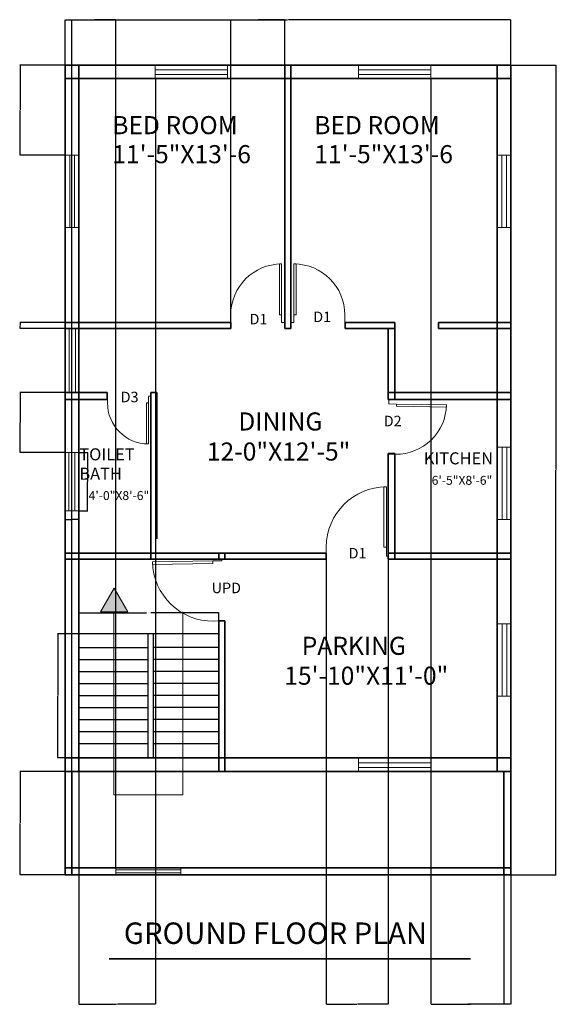
# Model space of a CAD drawing. Units: inches. Extents: x 2000 to 5103, y 1720 to 4295.
# Tile 1 of 2: x 2000 to 2357, y 1720 to 2374. Entities that reach past the tile are written whole.
import ezdxf

# ---------------------------------------------------------------- set-up
doc = ezdxf.new("R2010")
doc.units = ezdxf.units.IN
for name, color, linetype, lineweight in [('A-ANNO-DIMS', 2, 'Continuous', 18), ('A-ANNO-SYMB', 7, 'Continuous', 18), ('A-ANNO-TEXT', 3, 'Continuous', 18), ('A-ANNO-TITL', 7, 'Continuous', 35), ('A-AREA-IDEN', 7, 'Continuous', 25), ('A-DOOR', 4, 'Continuous', 18), ('A-WALL', 7, 'Continuous', 35), ('stair', 7, 'Continuous', 25), ('window', 10, 'Continuous', 18)]:
    doc.layers.add(name, color=color, linetype=linetype, lineweight=lineweight)
doc.styles.get("Standard").update_dxf_attribs({"font": 'arial.ttf'})
doc.dimstyles.get("Standard").update_dxf_attribs({"dimtxt": 0.18, "dimasz": 0.18, "dimexe": 0.18, "dimexo": 0.0625, "dimgap": 0.09, "dimtad": 0, "dimtih": 1, "dimtoh": 1, "dimdec": 4, "dimzin": 0, "dimdsep": 46, "dimtxsty": 'Standard', "dimcen": 0.09, "dimadec": 0, "dimazin": 0, "dimtfac": 1, "dimtdec": 4, "dimtofl": 0, "dimtmove": 0, "dimatfit": 3, "dimfxl": 1, "dimtolj": 1, "dimtzin": 0, "dimarcsym": 0})

# ---------------------------------------------------------------- blocks, each defined once
blk = doc.blocks.new('Dining Set - 36 x 72 in')
at = {"layer": 'window'}
for p, q in [((418.4, 887.02), (466.4, 887.02)), ((418.4, 883.92), (466.4, 883.92))]:
    blk.add_line(p, q, dxfattribs=at)
blk.add_lwpolyline([(418.4, 881.14), (418.4, 890.14), (466.4, 890.14), (466.4, 881.14)], close=True, dxfattribs=at)
blk = doc.blocks.new('*U3')
for p, q in [((0, 0), (0, -6)), ((40, 0), (40, -6))]:
    blk.add_line(p, q)
blk.add_lwpolyline([(0, 0), (0, 40), (1.75, 40), (1.75, 0)], close=True)
blk.add_arc((0, 0), 40, 0, 90)
blk = doc.blocks.new('WIN-DINING')
for p, q in [((2.68, 42.5), (2.68, 0)), ((4.5, 42.5), (4.5, 0)), ((6.78, 42.5), (6.78, 0))]:
    blk.add_line(p, q)
blk.add_lwpolyline([(0, 42.5), (9, 42.5), (9, 0), (0, 0)], close=True)
blk = doc.blocks.new('WIN-BATH')
for p, q in [((2.49, 38.59), (2.49, 0)), ((6.38, 38.59), (6.38, 0)), ((6.38, 38.59), (6.38, 0))]:
    blk.add_line(p, q)
blk.add_lwpolyline([(0, 38.59), (9, 38.59), (9, 0), (0, 0)], close=True)
blk = doc.blocks.new('WIN-FRONT')
for p, q in [((0, 3.25), (43.02, 3.25)), ((0, 1.25), (43.02, 1.25))]:
    blk.add_line(p, q)
blk.add_lwpolyline([(0, 4.5), (43.02, 4.5), (43.02, 0), (0, 0)], close=True)
blk = doc.blocks.new('STAIR-RETURN-FLIGHTS')
for p, q in [((93.06, 82.39), (0, 82.3)), ((46.1, 0), (46.1, 82.34)), ((49.5, 82.35), (49.5, 0)), ((0, 73.28), (46.1, 73.28)), ((49.5, 73.48), (93.06, 73.48)), ((49.5, 65.5), (93.06, 65.5)), ((0, 65.3), (46.1, 65.3)), ((0, 57.32), (46.1, 57.32)), ((49.5, 57.52), (93.06, 57.52)), ((0, 49.34), (46.1, 49.34)), ((49.5, 49.54), (93.06, 49.54)), ((0, 41.37), (46.1, 41.37)), ((49.5, 41.56), (93.06, 41.56)), ((0, 33.39), (46.1, 33.39)), ((49.5, 33.58), (93.06, 33.58)), ((0, 25.41), (46.1, 25.41)), ((49.5, 25.61), (93.06, 25.61)), ((0, 17.43), (46.1, 17.43)), ((49.5, 17.63), (93.06, 17.63)), ((0, 9.45), (46.1, 9.45)), ((49.5, 9.65), (93.06, 9.65))]:
    blk.add_line(p, q)
blk = doc.blocks.new('STAIR-PATH-ARROW')
h = blk.add_hatch(color=256)
h.dxf.hatch_style = 1
h.paths.add_polyline_path([(9.07, 137.14), (0, 121.43), (18.13, 121.43)])
for p, q in [((0, 121.43), (9.07, 137.14)), ((9.07, 137.14), (18.13, 121.43)), ((18.13, 121.43), (0, 121.43)), ((8.84, 0), (8.84, 121.43)), ((8.84, 121.43), (18.13, 121.43)), ((54.71, 121.43), (54.71, 0)), ((54.71, 0), (8.84, 0))]:
    blk.add_line(p, q)
blk = doc.blocks.new('*D13')
at = {"layer": 'A-ANNO-DIMS', "color": 0, "lineweight": -2, "transparency": 16777216}
for p, q in [((2039.72, 2086.19), (2045.62, 2086.19)), ((2045.44, 2086.01), (2045.44, 2067.07)), ((2045.44, 2047.77), (2045.44, 2066.71)), ((2039.72, 2047.59), (2045.62, 2047.59))]:
    blk.add_line(p, q, dxfattribs=at)
at = {"layer": 'A-ANNO-DIMS', "color": 0, "transparency": 16777216}
for points in [[(2045.41, 2086.01), (2045.47, 2086.01), (2045.44, 2086.19)], [(2045.41, 2047.77), (2045.47, 2047.77), (2045.44, 2047.59)]]:
    blk.add_solid(points, dxfattribs=at)
at = {"layer": 'Defpoints', "color": 0, "transparency": 16777216}
for p in [(2039.66, 2086.19), (2045.44, 2086.19), (2039.66, 2047.59)]:
    blk.add_point(p, dxfattribs=at)
at = {"layer": 'A-ANNO-DIMS', "color": 0, "transparency": 16777216, "insert": (2045.44, 2066.89), "char_height": 0.18, "attachment_point": 5}
blk.add_mtext('\\A1;WINDOW 39 TYP.', dxfattribs=at)
blk = doc.blocks.new('*D14')
at = {"layer": 'A-ANNO-DIMS', "color": 0, "lineweight": -2, "transparency": 16777216}
for p, q in [((2030.66, 2047.53), (2030.66, 2041.63)), ((2039.66, 2047.53), (2039.66, 2041.63)), ((2030.84, 2041.81), (2034.7, 2041.81)), ((2039.48, 2041.81), (2035.61, 2041.81))]:
    blk.add_line(p, q, dxfattribs=at)
at = {"layer": 'A-ANNO-DIMS', "color": 0, "transparency": 16777216}
for points in [[(2030.84, 2041.84), (2030.84, 2041.78), (2030.66, 2041.81)], [(2039.48, 2041.84), (2039.48, 2041.78), (2039.66, 2041.81)]]:
    blk.add_solid(points, dxfattribs=at)
at = {"layer": 'Defpoints', "color": 0, "transparency": 16777216}
for p in [(2030.66, 2047.59), (2039.66, 2047.59), (2039.66, 2041.81)]:
    blk.add_point(p, dxfattribs=at)
at = {"layer": 'A-ANNO-DIMS', "color": 0, "transparency": 16777216, "insert": (2035.16, 2041.81), "char_height": 0.18, "attachment_point": 5}
blk.add_mtext('\\A1;9 TYP.', dxfattribs=at)
blk = doc.blocks.new('*D17')
at = {"layer": 'A-ANNO-DIMS', "color": 0, "lineweight": -2, "transparency": 16777216}
for p, q in [((2039.66, 1965.97), (2039.66, 1980.04)), ((2039.84, 1979.86), (2084.7, 1979.86)), ((2132.54, 1979.86), (2087.67, 1979.86)), ((2132.72, 1965.97), (2132.72, 1980.04))]:
    blk.add_line(p, q, dxfattribs=at)
at = {"layer": 'A-ANNO-DIMS', "color": 0, "transparency": 16777216}
for points in [[(2039.84, 1979.89), (2039.84, 1979.83), (2039.66, 1979.86)], [(2132.54, 1979.89), (2132.54, 1979.83), (2132.72, 1979.86)]]:
    blk.add_solid(points, dxfattribs=at)
at = {"layer": 'Defpoints', "color": 0, "transparency": 16777216}
for p in [(2132.72, 1979.86), (2039.66, 1965.9), (2132.72, 1965.9)]:
    blk.add_point(p, dxfattribs=at)
at = {"layer": 'A-ANNO-DIMS', "color": 0, "transparency": 16777216, "insert": (2086.19, 1979.86), "char_height": 0.18, "attachment_point": 5}
blk.add_mtext('\\A1;RETURN STAIR 93 TYP.', dxfattribs=at)
blk = doc.blocks.new('*D18')
at = {"layer": 'A-ANNO-DIMS', "color": 0, "lineweight": -2, "transparency": 16777216}
for p, q in [((2039.59, 1965.9), (2025.52, 1965.9)), ((2025.7, 1965.72), (2025.7, 1924.89)), ((2025.7, 1883.69), (2025.7, 1924.53)), ((2039.59, 1883.51), (2025.52, 1883.51))]:
    blk.add_line(p, q, dxfattribs=at)
at = {"layer": 'A-ANNO-DIMS', "color": 0, "transparency": 16777216}
for points in [[(2025.67, 1965.72), (2025.73, 1965.72), (2025.7, 1965.9)], [(2025.67, 1883.69), (2025.73, 1883.69), (2025.7, 1883.51)]]:
    blk.add_solid(points, dxfattribs=at)
at = {"layer": 'Defpoints', "color": 0, "transparency": 16777216}
for p in [(2025.7, 1965.9), (2039.66, 1965.9), (2039.66, 1883.51)]:
    blk.add_point(p, dxfattribs=at)
at = {"layer": 'A-ANNO-DIMS', "color": 0, "transparency": 16777216, "insert": (2025.7, 1924.71), "char_height": 0.18, "attachment_point": 5}
blk.add_mtext('\\A1;82 TYP.', dxfattribs=at)
blk = doc.blocks.new('*D19')
at = {"layer": 'A-ANNO-DIMS', "color": 0, "lineweight": -2, "transparency": 16777216}
for p, q in [((2030.66, 2343.57), (2030.66, 2373.59)), ((2030.84, 2373.41), (2178.37, 2373.41)), ((2326.48, 2373.41), (2178.95, 2373.41)), ((2326.66, 2343.57), (2326.66, 2373.59))]:
    blk.add_line(p, q, dxfattribs=at)
at = {"layer": 'A-ANNO-DIMS', "color": 0, "transparency": 16777216}
for points in [[(2030.84, 2373.44), (2030.84, 2373.38), (2030.66, 2373.41)], [(2326.48, 2373.44), (2326.48, 2373.38), (2326.66, 2373.41)]]:
    blk.add_solid(points, dxfattribs=at)
at = {"layer": 'Defpoints', "color": 0, "transparency": 16777216}
for p in [(2326.66, 2373.41), (2030.66, 2343.51), (2326.66, 2343.51)]:
    blk.add_point(p, dxfattribs=at)
at = {"layer": 'A-ANNO-DIMS', "color": 0, "transparency": 16777216, "insert": (2178.66, 2373.41), "char_height": 0.18, "attachment_point": 5}
blk.add_mtext('\\A1;296', dxfattribs=at)
blk = doc.blocks.new('*D20')
at = {"layer": 'A-ANNO-DIMS', "color": 0, "lineweight": -2, "transparency": 16777216}
for p, q in [((2326.72, 2343.51), (2356.85, 2343.51)), ((2356.67, 2343.33), (2356.67, 2074.9)), ((2356.67, 1806.1), (2356.67, 2074.54)), ((2326.72, 1805.92), (2356.85, 1805.92))]:
    blk.add_line(p, q, dxfattribs=at)
at = {"layer": 'A-ANNO-DIMS', "color": 0, "transparency": 16777216}
for points in [[(2356.64, 2343.33), (2356.7, 2343.33), (2356.67, 2343.51)], [(2356.64, 1806.1), (2356.7, 1806.1), (2356.67, 1805.92)]]:
    blk.add_solid(points, dxfattribs=at)
at = {"layer": 'Defpoints', "color": 0, "transparency": 16777216}
for p in [(2326.66, 2343.51), (2356.67, 2343.51), (2326.66, 1805.92)]:
    blk.add_point(p, dxfattribs=at)
at = {"layer": 'A-ANNO-DIMS', "color": 0, "transparency": 16777216, "insert": (2356.67, 2074.72), "char_height": 0.18, "attachment_point": 5}
blk.add_mtext('\\A1;537.6', dxfattribs=at)
blk = doc.blocks.new('*D23')
at = {"layer": 'A-ANNO-DIMS', "color": 0, "lineweight": -2, "transparency": 16777216}
for p, q in [((2030.59, 1874.51), (2000.58, 1874.51)), ((2000.76, 1874.33), (2000.76, 1840.4)), ((2000.76, 1806.1), (2000.76, 1840.04)), ((2030.59, 1805.92), (2000.58, 1805.92))]:
    blk.add_line(p, q, dxfattribs=at)
at = {"layer": 'A-ANNO-DIMS', "color": 0, "transparency": 16777216}
for points in [[(2000.73, 1874.33), (2000.79, 1874.33), (2000.76, 1874.51)], [(2000.73, 1806.1), (2000.79, 1806.1), (2000.76, 1805.92)]]:
    blk.add_solid(points, dxfattribs=at)
at = {"layer": 'Defpoints', "color": 0, "transparency": 16777216}
for p in [(2000.76, 1874.51), (2030.66, 1874.51), (2030.66, 1805.92)]:
    blk.add_point(p, dxfattribs=at)
at = {"layer": 'A-ANNO-DIMS', "color": 0, "transparency": 16777216, "insert": (2000.76, 1840.22), "char_height": 0.18, "attachment_point": 5}
blk.add_mtext('\\A1;68.59', dxfattribs=at)
blk = doc.blocks.new('*D24')
at = {"layer": 'A-ANNO-DIMS', "color": 0, "lineweight": -2, "transparency": 16777216}
for p, q in [((2030.59, 2343.51), (2000.58, 2343.51)), ((2000.76, 2343.33), (2000.76, 2313.76)), ((2000.76, 2283.83), (2000.76, 2313.4)), ((2030.59, 2283.65), (2000.58, 2283.65))]:
    blk.add_line(p, q, dxfattribs=at)
at = {"layer": 'A-ANNO-DIMS', "color": 0, "transparency": 16777216}
for points in [[(2000.73, 2343.33), (2000.79, 2343.33), (2000.76, 2343.51)], [(2000.73, 2283.83), (2000.79, 2283.83), (2000.76, 2283.65)]]:
    blk.add_solid(points, dxfattribs=at)
at = {"layer": 'Defpoints', "color": 0, "transparency": 16777216}
for p in [(2030.66, 2343.51), (2000.76, 2283.65), (2030.66, 2283.65)]:
    blk.add_point(p, dxfattribs=at)
at = {"layer": 'A-ANNO-DIMS', "color": 0, "transparency": 16777216, "insert": (2000.76, 2313.58), "char_height": 0.18, "attachment_point": 5}
blk.add_mtext('\\A1;59.86', dxfattribs=at)
blk = doc.blocks.new('*D25')
at = {"layer": 'A-ANNO-DIMS', "color": 0, "lineweight": -2, "transparency": 16777216}
for p, q in [((2030.59, 2126.01), (2000.58, 2126.01)), ((2000.76, 2125.83), (2000.76, 2106.28)), ((2000.76, 2086.37), (2000.76, 2105.92)), ((2030.59, 2086.19), (2000.58, 2086.19))]:
    blk.add_line(p, q, dxfattribs=at)
at = {"layer": 'A-ANNO-DIMS', "color": 0, "transparency": 16777216}
for points in [[(2000.73, 2125.83), (2000.79, 2125.83), (2000.76, 2126.01)], [(2000.73, 2086.37), (2000.79, 2086.37), (2000.76, 2086.19)]]:
    blk.add_solid(points, dxfattribs=at)
at = {"layer": 'Defpoints', "color": 0, "transparency": 16777216}
for p in [(2030.66, 2126.01), (2000.76, 2086.19), (2030.66, 2086.19)]:
    blk.add_point(p, dxfattribs=at)
at = {"layer": 'A-ANNO-DIMS', "color": 0, "transparency": 16777216, "insert": (2000.76, 2106.1), "char_height": 0.18, "attachment_point": 5}
blk.add_mtext('\\A1;39.83', dxfattribs=at)
blk = doc.blocks.new('*D26')
at = {"layer": 'A-ANNO-DIMS', "color": 0, "lineweight": -2, "transparency": 16777216}
for p, q in [((2035.16, 1805.99), (2035.16, 2373.59)), ((2035.34, 2373.41), (2049.39, 2373.41)), ((2064.24, 2373.41), (2050.18, 2373.41)), ((2064.42, 1810.49), (2064.42, 2373.59))]:
    blk.add_line(p, q, dxfattribs=at)
at = {"layer": 'A-ANNO-DIMS', "color": 0, "transparency": 16777216}
for points in [[(2035.34, 2373.44), (2035.34, 2373.38), (2035.16, 2373.41)], [(2064.24, 2373.44), (2064.24, 2373.38), (2064.42, 2373.41)]]:
    blk.add_solid(points, dxfattribs=at)
at = {"layer": 'Defpoints', "color": 0, "transparency": 16777216}
for p in [(2064.42, 2373.41), (2035.16, 1805.92), (2064.42, 1810.42)]:
    blk.add_point(p, dxfattribs=at)
at = {"layer": 'A-ANNO-DIMS', "color": 0, "transparency": 16777216, "insert": (2049.79, 2373.41), "char_height": 0.18, "attachment_point": 5}
blk.add_mtext('\\A1;29.26', dxfattribs=at)
blk = doc.blocks.new('*D27')
at = {"layer": 'A-ANNO-DIMS', "color": 0, "lineweight": -2, "transparency": 16777216}
for p, q in [((2039.66, 2343.45), (2039.66, 1719.92)), ((2090.58, 2334.45), (2090.58, 1719.92)), ((2039.84, 1720.1), (2064.72, 1720.1)), ((2090.4, 1720.1), (2065.51, 1720.1))]:
    blk.add_line(p, q, dxfattribs=at)
at = {"layer": 'A-ANNO-DIMS', "color": 0, "transparency": 16777216}
for points in [[(2039.84, 1720.13), (2039.84, 1720.07), (2039.66, 1720.1)], [(2090.4, 1720.13), (2090.4, 1720.07), (2090.58, 1720.1)]]:
    blk.add_solid(points, dxfattribs=at)
at = {"layer": 'Defpoints', "color": 0, "transparency": 16777216}
for p in [(2039.66, 2343.51), (2090.58, 2334.51), (2090.58, 1720.1)]:
    blk.add_point(p, dxfattribs=at)
at = {"layer": 'A-ANNO-DIMS', "color": 0, "transparency": 16777216, "insert": (2065.12, 1720.1), "char_height": 0.18, "attachment_point": 5}
blk.add_mtext('\\A1;50.92', dxfattribs=at)
blk = doc.blocks.new('*D28')
at = {"layer": 'A-ANNO-DIMS', "color": 0, "lineweight": -2, "transparency": 16777216}
for p, q in [((2273.66, 2334.45), (2273.66, 1719.92)), ((2326.66, 2334.45), (2326.66, 1719.92)), ((2273.84, 1720.1), (2299.94, 1720.1)), ((2326.48, 1720.1), (2300.37, 1720.1))]:
    blk.add_line(p, q, dxfattribs=at)
at = {"layer": 'A-ANNO-DIMS', "color": 0, "transparency": 16777216}
for points in [[(2273.84, 1720.13), (2273.84, 1720.07), (2273.66, 1720.1)], [(2326.48, 1720.13), (2326.48, 1720.07), (2326.66, 1720.1)]]:
    blk.add_solid(points, dxfattribs=at)
at = {"layer": 'Defpoints', "color": 0, "transparency": 16777216}
for p in [(2273.66, 2334.51), (2326.66, 2334.51), (2326.66, 1720.1)]:
    blk.add_point(p, dxfattribs=at)
at = {"layer": 'A-ANNO-DIMS', "color": 0, "transparency": 16777216, "insert": (2300.16, 1720.1), "char_height": 0.18, "attachment_point": 5}
blk.add_mtext('\\A1;53', dxfattribs=at)
blk = doc.blocks.new('*D31')
at = {"layer": 'A-ANNO-DIMS', "color": 0, "lineweight": -2, "transparency": 16777216}
for p, q in [((2273.66, 1874.36), (2273.66, 1719.92)), ((2322.16, 1874.45), (2322.16, 1719.92)), ((2273.84, 1720.1), (2297.58, 1720.1)), ((2321.98, 1720.1), (2298.23, 1720.1))]:
    blk.add_line(p, q, dxfattribs=at)
at = {"layer": 'A-ANNO-DIMS', "color": 0, "transparency": 16777216}
for points in [[(2273.84, 1720.13), (2273.84, 1720.07), (2273.66, 1720.1)], [(2321.98, 1720.13), (2321.98, 1720.07), (2322.16, 1720.1)]]:
    blk.add_solid(points, dxfattribs=at)
at = {"layer": 'Defpoints', "color": 0, "transparency": 16777216}
for p in [(2273.66, 1874.42), (2322.16, 1874.51), (2273.66, 1720.1)]:
    blk.add_point(p, dxfattribs=at)
at = {"layer": 'A-ANNO-DIMS', "color": 0, "transparency": 16777216, "insert": (2297.91, 1720.1), "char_height": 0.18, "attachment_point": 5}
blk.add_mtext('\\A1;48.5', dxfattribs=at)
blk = doc.blocks.new('*D34')
at = {"layer": 'A-ANNO-DIMS', "color": 0, "lineweight": -2, "transparency": 16777216}
for p, q in [((2140.66, 2168.57), (2140.66, 2373.59)), ((2140.84, 2373.41), (2158.44, 2373.41)), ((2176.48, 2373.41), (2158.87, 2373.41)), ((2176.66, 2168.57), (2176.66, 2373.59))]:
    blk.add_line(p, q, dxfattribs=at)
at = {"layer": 'A-ANNO-DIMS', "color": 0, "transparency": 16777216}
for points in [[(2140.84, 2373.44), (2140.84, 2373.38), (2140.66, 2373.41)], [(2176.48, 2373.44), (2176.48, 2373.38), (2176.66, 2373.41)]]:
    blk.add_solid(points, dxfattribs=at)
at = {"layer": 'Defpoints', "color": 0, "transparency": 16777216}
for p in [(2176.66, 2373.41), (2140.66, 2168.51), (2176.66, 2168.51)]:
    blk.add_point(p, dxfattribs=at)
at = {"layer": 'A-ANNO-DIMS', "color": 0, "transparency": 16777216, "insert": (2158.66, 2373.41), "char_height": 0.18, "attachment_point": 5}
blk.add_mtext('\\A1;36', dxfattribs=at)
blk = doc.blocks.new('*D35')
at = {"layer": 'A-ANNO-DIMS', "color": 0, "lineweight": -2, "transparency": 16777216}
for p, q in [((2204.16, 2015.45), (2204.16, 1719.92)), ((2245.16, 2015.45), (2245.16, 1719.92)), ((2204.34, 1720.1), (2224.45, 1720.1)), ((2244.98, 1720.1), (2224.86, 1720.1))]:
    blk.add_line(p, q, dxfattribs=at)
at = {"layer": 'A-ANNO-DIMS', "color": 0, "transparency": 16777216}
for points in [[(2204.34, 1720.13), (2204.34, 1720.07), (2204.16, 1720.1)], [(2244.98, 1720.13), (2244.98, 1720.07), (2245.16, 1720.1)]]:
    blk.add_solid(points, dxfattribs=at)
at = {"layer": 'Defpoints', "color": 0, "transparency": 16777216}
for p in [(2204.16, 2015.51), (2245.16, 2015.51), (2245.16, 1720.1)]:
    blk.add_point(p, dxfattribs=at)
at = {"layer": 'A-ANNO-DIMS', "color": 0, "transparency": 16777216, "insert": (2224.66, 1720.1), "char_height": 0.18, "attachment_point": 5}
blk.add_mtext('\\A1;41', dxfattribs=at)
blk = doc.blocks.new('*D38')
at = {"layer": 'A-ANNO-DIMS', "color": 0, "lineweight": -2, "transparency": 16777216}
for p, q in [((2030.593513, 2172.511961), (2000.576013, 2172.511961)), ((2000.756013, 2172.331961), (2000.756013, 2170.691961)), ((2000.756013, 2168.691961), (2000.756013, 2170.331961)), ((2030.593513, 2168.511961), (2000.576013, 2168.511961))]:
    blk.add_line(p, q, dxfattribs=at)
at = {"layer": 'A-ANNO-DIMS', "color": 0, "transparency": 16777216}
for points in [[(2000.726013, 2172.331961), (2000.786013, 2172.331961), (2000.756013, 2172.511961)], [(2000.726013, 2168.691961), (2000.786013, 2168.691961), (2000.756013, 2168.511961)]]:
    blk.add_solid(points, dxfattribs=at)
at = {"layer": 'Defpoints', "color": 0, "transparency": 16777216}
for p in [(2000.756013, 2172.511961), (2030.656013, 2172.511961), (2030.656013, 2168.511961)]:
    blk.add_point(p, dxfattribs=at)
at = {"layer": 'A-ANNO-DIMS', "color": 0, "transparency": 16777216, "insert": (2000.756013, 2170.511961), "char_height": 0.18, "attachment_point": 5}
blk.add_mtext('\\A1;4', dxfattribs=at)

msp = doc.modelspace()

# ---------------------------------------------------------------- linework, layer by layer
at = {"layer": 'A-ANNO-TITL'}
msp.add_line((2060, 1750), (2300, 1750), dxfattribs=at)
at = {"layer": 'A-DOOR'}
for p, q in [((2174.4791, 2172.512), (2176.656, 2172.512)), ((2182.644, 2172.512), (2180.656, 2172.512)), ((2086.0849, 2123.5546), (2087.656, 2123.5546)), ((2245.7341, 2118.4632), (2245.7341, 2121.512)), ((2134.7166, 2014.3573), (2134.7166, 2015.512)), ((2244.1241, 2017.512), (2245.156, 2017.512))]:
    msp.add_line(p, q, dxfattribs=at)
at = {"layer": 'A-WALL'}
for p, q in [((2030.656, 2343.512), (2030.656, 1874.512)), ((2030.656, 2343.512), (2326.656, 2343.512)), ((2039.656, 2343.512), (2039.656, 1874.512)), ((2176.656, 2343.512), (2176.656, 2168.512)), ((2180.656, 2343.512), (2180.656, 2168.512)), ((2317.656, 2343.512), (2317.656, 1874.512)), ((2326.656, 2343.512), (2326.656, 1874.512)), ((2030.656, 2334.512), (2326.656, 2334.512)), ((2030.656, 2172.512), (2140.656, 2172.512)), ((2140.656, 2168.512), (2140.656, 2172.512)), ((2216.656, 2172.512), (2249.656, 2172.512)), ((2216.656, 2168.512), (2216.656, 2172.512)), ((2249.656, 2172.512), (2249.656, 2121.512)), ((2278.656, 2172.512), (2326.656, 2172.512)), ((2278.656, 2168.512), (2278.656, 2172.512)), ((2030.656, 2168.512), (2140.656, 2168.512)), ((2176.656, 2168.512), (2180.656, 2168.512)), ((2216.656, 2168.512), (2249.656, 2168.512)), ((2245.156, 2168.512), (2245.156, 2121.512)), ((2278.656, 2168.512), (2326.656, 2168.512)), ((2030.656, 2126.012), (2058.656, 2126.012)), ((2058.656, 2121.512), (2058.656, 2126.012)), ((2087.656, 2126.012), (2087.656, 2015.512)), ((2087.656, 2126.012), (2091.5827, 2126.012)), ((2091.5827, 2126.012), (2091.5827, 2029.0177)), ((2245.156, 2126.012), (2326.656, 2126.012)), ((2030.656, 2121.512), (2058.656, 2121.512)), ((2245.156, 2121.512), (2326.656, 2121.512)), ((2245.156, 2085.512), (2245.156, 2015.512)), ((2249.656, 2085.512), (2245.156, 2085.512)), ((2249.656, 2085.512), (2249.656, 2015.512)), ((2030.656, 2019.512), (2204.156, 2019.512)), ((2030.656, 2015.512), (2204.156, 2015.512)), ((2132.7166, 2019.512), (2132.7166, 2015.512)), ((2136.7166, 2019.512), (2136.7166, 2015.512)), ((2204.156, 2015.512), (2204.156, 2019.512)), ((2245.156, 2019.512), (2326.656, 2019.512)), ((2245.156, 2015.512), (2326.656, 2015.512)), ((2245.156, 2015.512), (2245.156, 2015.512)), ((2132.7166, 1974.512), (2132.7166, 1874.512)), ((2136.7166, 1974.512), (2132.7166, 1974.512)), ((2136.7166, 1974.512), (2136.7166, 1874.512)), ((2030.656, 1883.512), (2326.656, 1883.512)), ((2030.656, 1874.512), (2326.656, 1874.512)), ((2030.656, 1874.512), (2030.656, 1805.9232)), ((2035.156, 1874.512), (2035.156, 1805.9232)), ((2322.156, 1805.9232), (2322.156, 1874.512)), ((2326.656, 1805.9232), (2326.656, 1874.512)), ((2030.656, 1810.4232), (2326.656, 1810.4232)), ((2030.656, 1805.9232), (2326.656, 1805.9232))]:
    msp.add_line(p, q, dxfattribs=at)

# ---------------------------------------------------------------- block references
at = {"layer": 'A-ANNO-SYMB'}
msp.add_blockref('STAIR-PATH-ARROW', (2054.0769, 1859.0751), dxfattribs=at)
at = {"layer": 'A-DOOR'}
for p, xscale, yscale, zscale in [((2174.4791, 2177.5854), -0.8455769532508881, 0.8455769532508881, 0.8455769532508881), ((2182.644, 2177.5854), 0.8455769532508881, 0.8455769532508881, 0.8455769532508881), ((2244.1241, 2023.5072), -0.9992024495959569, 0.9992024495959569, 0.9992024495959569)]:
    msp.add_blockref('*U3', p, dxfattribs=dict(at, xscale=xscale, yscale=yscale, zscale=zscale))
for p, xscale, yscale, zscale, rotation in [((2085.9845, 2119.1275), 0.680435440491929, 0.680435440491929, 0.680435440491929, 180), ((2250.7216, 2118.3911), 0.8313368246920212, 0.8313368246920212, 0.8313368246920212, 269.1712141329585), ((2128.722, 2014.2705), -0.9992024495959569, 0.9992024495959569, 0.9992024495959569, 90.82878586703616)]:
    msp.add_blockref('*U3', p, dxfattribs=dict(at, xscale=xscale, yscale=yscale, zscale=zscale, rotation=rotation))
at = {"layer": 'stair'}
msp.add_blockref('STAIR-RETURN-FLIGHTS', (2039.656, 1883.512), dxfattribs=at)
at = {"layer": 'window'}
for name, p in [('Dining Set - 36 x 72 in', (1672.1725, 1453.3734)), ('Dining Set - 36 x 72 in', (1807.2517, 1453.3734)), ('WIN-DINING', (2030.656, 2126.012)), ('WIN-BATH', (2030.656, 2047.594)), ('Dining Set - 36 x 72 in', (1807.2517, 993.2789)), ('WIN-FRONT', (2064.4157, 1805.9232))]:
    msp.add_blockref(name, p, dxfattribs=at)
at = {"layer": 'window', "rotation": 90}
for p in [(2920.7946, 1817.2445), (3207.7851, 1817.2445), (3207.9134, 1623.3945), (3207.9134, 1506.0077)]:
    msp.add_blockref('Dining Set - 36 x 72 in', p, dxfattribs=at)

# ---------------------------------------------------------------- texts
at = {"layer": 'A-ANNO-DIMS'}
for s, height, p in [('11\'-5"X13\'-6', 12, (2061.9802, 2278.3157)), ('11\'-5"X13\'-6', 12, (2196.1844, 2278.3157)), ('12-0"X12\'-5"', 12, (2124.7896, 2080.9095)), ('6\'-5"X8\'-6"', 5.914719, (2274.1708, 2064.8269)), ('4\'-0"X8\'-6"', 5.914719, (2046.2547, 2054.7138)), ('15\'-10"X11\'-0"', 12, (2176.2252, 1932.0818))]:
    msp.add_text(s, height=height, dxfattribs=at).set_placement(p)
at = {"layer": 'A-ANNO-TEXT'}
for s, p in [('D1', (2153.176, 2171.3142)), ('D1', (2195.4906, 2172.8057)), ('D3', (2067.551, 2119.606)), ('D2', (2242.3148, 2103.654)), ('D1', (2219.0044, 2015.9242)), ('UPD', (2127.9989, 1992.857))]:
    msp.add_text(s, height=7, dxfattribs=at).set_placement(p)
at = {"layer": 'A-ANNO-TITL'}
msp.add_text('GROUND FLOOR PLAN', height=14.242438, dxfattribs=at).set_placement((2069.6537, 1760))
at = {"layer": 'A-AREA-IDEN'}
for s, height, p in [('BED ROOM', 12, (2061.9802, 2297.5927)), ('BED ROOM', 12, (2196.1844, 2297.5927)), ('DINING', 12, (2145.7298, 2100.8611)), ('TOILET', 8, (2040.0843, 2081.0319)), ('KITCHEN', 8, (2268.9504, 2078.3895)), ('BATH', 8, (2040.0843, 2068.1806)), ('PARKING', 12, (2187.8424, 1951.9113))]:
    msp.add_text(s, height=height, dxfattribs=at).set_placement(p)

# ---------------------------------------------------------------- dimensions: what is measured, and where the dimension line sits
at = {"layer": 'A-ANNO-DIMS'}
for base, p1, p2, override, picture, middle in [((2326.656, 2373.412), (2030.656, 2343.512), (2326.656, 2343.512), {"dimdec": 0, "dimlfac": 1, "dimrnd": 0, "dimzin": 0, "dimdsep": 46, "dimlunit": 2}, '*D19', (2178.656, 2373.412)), ((2064.4157, 2373.412), (2035.156, 1805.9232), (2064.4157, 1810.4232), {"dimdec": 2, "dimlfac": 1, "dimrnd": 0, "dimzin": 0, "dimdsep": 46, "dimlunit": 2}, '*D26', (2049.7858, 2373.412)), ((2176.656, 2373.412), (2140.656, 2168.512), (2176.656, 2168.512), {"dimdec": 0, "dimlfac": 1, "dimrnd": 0, "dimzin": 0, "dimdsep": 46, "dimlunit": 2}, '*D34', (2158.656, 2373.412)), ((2090.5768, 1720.1), (2039.656, 2343.512), (2090.5768, 2334.512), {"dimdec": 2, "dimlfac": 1, "dimrnd": 0, "dimzin": 0, "dimdsep": 46, "dimlunit": 2}, '*D27', (2065.1164, 1720.1)), ((2326.656, 1720.1), (2273.656, 2334.512), (2326.656, 2334.512), {"dimdec": 0, "dimlfac": 1, "dimrnd": 0, "dimzin": 0, "dimdsep": 46, "dimlunit": 2}, '*D28', (2300.156, 1720.1)), ((2245.156, 1720.1), (2204.156, 2015.512), (2245.156, 2015.512), {"dimdec": 0, "dimlfac": 1, "dimrnd": 0, "dimzin": 0, "dimdsep": 46, "dimlunit": 2}, '*D35', (2224.656, 1720.1)), ((2273.656, 1720.1), (2322.156, 1874.512), (2273.656, 1874.4175), {"dimdec": 1, "dimlfac": 1, "dimrnd": 0, "dimzin": 0, "dimdsep": 46, "dimlunit": 2}, '*D31', (2297.906, 1720.1))]:
    dim = msp.add_linear_dim(base=base, p1=p1, p2=p2, dimstyle='Standard', override=override, dxfattribs=at)
    dim.commit()
    dim.dimension.update_dxf_attribs({"geometry": picture, "text_midpoint": middle})
for base, p1, p2, override, picture, middle in [((2000.756, 2283.6488), (2030.656, 2343.512), (2030.656, 2283.6488), {"dimdec": 2, "dimlfac": 1, "dimrnd": 0, "dimzin": 0, "dimdsep": 46, "dimlunit": 2}, '*D24', (2000.756, 2313.5804)), ((2356.6748, 2343.512), (2326.656, 1805.9232), (2326.656, 2343.512), {"dimdec": 1, "dimlfac": 1, "dimrnd": 0, "dimzin": 0, "dimdsep": 46, "dimlunit": 2}, '*D20', (2356.6748, 2074.7176)), ((2000.756, 2172.512), (2030.656, 2168.512), (2030.656, 2172.512), {"dimdec": 0, "dimlfac": 1, "dimrnd": 0, "dimzin": 0, "dimdsep": 46, "dimlunit": 2}, '*D38', (2000.756, 2170.512)), ((2000.756, 2086.1858), (2030.656, 2126.012), (2030.656, 2086.1858), {"dimdec": 2, "dimlfac": 1, "dimrnd": 0, "dimzin": 0, "dimdsep": 46, "dimlunit": 2}, '*D25', (2000.756, 2106.0989)), ((2000.756, 1874.512), (2030.656, 1805.9232), (2030.656, 1874.512), {"dimdec": 2, "dimlfac": 1, "dimrnd": 0, "dimzin": 0, "dimdsep": 46, "dimlunit": 2}, '*D23', (2000.756, 1840.2176))]:
    dim = msp.add_linear_dim(base=base, p1=p1, p2=p2, angle=90, dimstyle='Standard', override=override, dxfattribs=at)
    dim.commit()
    dim.dimension.update_dxf_attribs({"geometry": picture, "text_midpoint": middle})
for base, p1, p2, text, picture, middle in [((2045.4448, 2086.1858), (2039.656, 2047.594), (2039.656, 2086.1858), 'WINDOW <> TYP.', '*D13', (2045.4448, 2066.8899)), ((2025.6969, 1965.9027), (2039.656, 1883.512), (2039.656, 1965.9027), '<> TYP.', '*D18', (2025.6969, 1924.7073))]:
    dim = msp.add_linear_dim(base=base, p1=p1, p2=p2, angle=90, text=text, dimstyle='Standard', override={"dimdec": 0, "dimlfac": 1, "dimrnd": 0, "dimzin": 0, "dimdsep": 46, "dimlunit": 2}, dxfattribs=at)
    dim.commit()
    dim.dimension.update_dxf_attribs({"geometry": picture, "text_midpoint": middle})
for base, p1, p2, text, picture, middle in [((2039.656, 2041.8052), (2030.656, 2047.594), (2039.656, 2047.594), '<> TYP.', '*D14', (2035.156, 2041.8052)), ((2132.7166, 1979.8618), (2039.656, 1965.9027), (2132.7166, 1965.9027), 'RETURN STAIR <> TYP.', '*D17', (2086.1863, 1979.8618))]:
    dim = msp.add_linear_dim(base=base, p1=p1, p2=p2, text=text, dimstyle='Standard', override={"dimdec": 0, "dimlfac": 1, "dimrnd": 0, "dimzin": 0, "dimdsep": 46, "dimlunit": 2}, dxfattribs=at)
    dim.commit()
    dim.dimension.update_dxf_attribs({"geometry": picture, "text_midpoint": middle})

doc.saveas('drawing.dxf')
